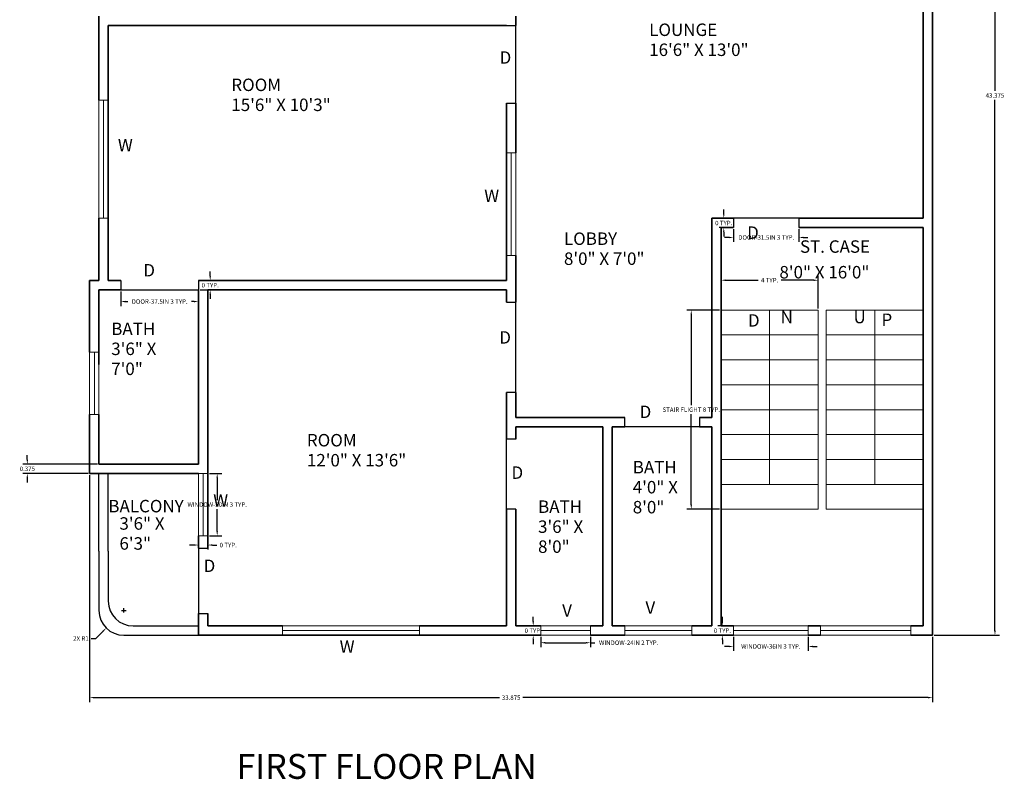
# Model space of a CAD drawing. Units: feet. Extents: x 60.2 to 151.6, y 170.7 to 222.6.
# Tile 2 of 3: x 112 to 151.6, y 170.7 to 201.2. Entities that reach past the tile are written whole.
import ezdxf

# ---------------------------------------------------------------- set-up
doc = ezdxf.new("R2010")
doc.units = ezdxf.units.FT
for name, color, linetype, lineweight in [('A-ANNO-DIMS', 7, 'Continuous', 13), ('A-ANNO-TEXT', 7, 'Continuous', 13), ('A-ANNO-TITL', 7, 'Continuous', 25), ('A-AREA-IDEN', 7, 'Continuous', 18), ('A-DOOR', 6, 'Continuous', 25), ('A-FLOR-BALC', 6, 'Continuous', 25), ('A-FLOR-STRS', 6, 'Continuous', 18), ('A-GLAZ', 240, 'Continuous', 18), ('A-WALL', 175, 'Continuous', 35)]:
    doc.layers.add(name, color=color, linetype=linetype, lineweight=lineweight)
doc.styles.get("Standard").update_dxf_attribs({"font": 'arial.ttf'})
doc.dimstyles.get("Standard").update_dxf_attribs({"dimtxt": 0.18, "dimasz": 0.18, "dimexe": 0.18, "dimexo": 0.0625, "dimgap": 0.09, "dimtad": 0, "dimtih": 1, "dimtoh": 1, "dimdec": 4, "dimzin": 0, "dimdsep": 46, "dimtxsty": 'Standard', "dimcen": 0.09, "dimadec": 0, "dimazin": 0, "dimtfac": 1, "dimtdec": 4, "dimtofl": 0, "dimtmove": 0, "dimatfit": 3, "dimfxl": 1, "dimtolj": 1, "dimtzin": 0, "dimarcsym": 0})

# ---------------------------------------------------------------- blocks, each defined once
blk = doc.blocks.new('DOOR-36IN')
for p, q in [((0, 0.375), (3, 0.375)), ((0, 0), (0, 0.375)), ((3, 0.375), (3, 0))]:
    blk.add_line(p, q)
blk = doc.blocks.new('DOOR-31_5IN')
for p, q in [((0, 2.625), (0, 0)), ((0, 2.625), (0.375, 2.625)), ((0, 0), (0.375, 0))]:
    blk.add_line(p, q)
blk = doc.blocks.new('DOOR-37_5IN')
for p, q in [((0, 0.375), (0, 0)), ((0, 0), (3.125, 0)), ((3.125, 0.375), (3.125, 0))]:
    blk.add_line(p, q)
blk = doc.blocks.new('WINDOW-24IN')
for p, q in [((0, 2), (0.375, 2)), ((0, 2), (0, 0)), ((0.188, 2), (0.188, 0)), ((0.375, 2), (0.375, 0)), ((0, 0), (0.375, 0))]:
    blk.add_line(p, q)
blk = doc.blocks.new('WINDOW-66IN')
for p, q in [((0.375, 5.5), (0, 5.5)), ((0, 0), (0, 5.5)), ((0.188, 5.5), (0.188, 0)), ((0.375, 0), (0.375, 5.5)), ((0.375, 0), (0, 0))]:
    blk.add_line(p, q)
blk = doc.blocks.new('WINDOW-30IN')
for p, q in [((0, 2.5), (0, 0)), ((0, 2.5), (0.375, 2.5)), ((0.188, 2.5), (0.188, 0)), ((0.375, 2.5), (0.375, 0)), ((0.375, 0.5), (0.375, 0)), ((0.375, 0), (0, 0))]:
    blk.add_line(p, q)
blk = doc.blocks.new('STAIR-FLIGHT-9-TREADS')
for p, q in [((0, 8), (3.9, 8)), ((1.95, 8), (1.95, 1)), ((3.9, 8), (3.9, 0)), ((0, 7), (3.9, 7)), ((0, 6), (3.9, 6)), ((0, 5), (3.9, 5)), ((0, 4), (3.9, 4)), ((0, 3), (3.9, 3)), ((0, 2), (3.9, 2)), ((0, 1), (3.9, 1)), ((0, 0), (3.9, 0))]:
    blk.add_line(p, q)
blk = doc.blocks.new('WINDOW-36IN')
for p, q in [((0, 0), (0, 3)), ((0, 3), (0.375, 3)), ((0.188, 3), (0.188, 0)), ((0.375, 3), (0.375, 0)), ((0.375, 0), (0, 0))]:
    blk.add_line(p, q)
blk = doc.blocks.new('*D20')
at = {"layer": 'A-ANNO-DIMS', "color": 0, "lineweight": -2, "transparency": 16777216}
for p, q in [((140.714, 192.831), (140.714, 192.319)), ((143.339, 192.831), (143.339, 192.319)), ((140.534, 192.499), (140.354, 192.499)), ((143.519, 192.499), (143.699, 192.499))]:
    blk.add_line(p, q, dxfattribs=at)
at = {"layer": 'A-ANNO-DIMS', "color": 0, "transparency": 16777216}
for points in [[(140.534, 192.529), (140.534, 192.469), (140.714, 192.499)], [(143.519, 192.529), (143.519, 192.469), (143.339, 192.499)]]:
    blk.add_solid(points, dxfattribs=at)
at = {"layer": 'Defpoints', "color": 0, "transparency": 16777216}
for p in [(140.714, 192.893), (143.339, 192.893), (143.339, 192.499)]:
    blk.add_point(p, dxfattribs=at)
at = {"layer": 'A-ANNO-DIMS', "color": 0, "transparency": 16777216, "insert": (142.027, 192.499), "char_height": 0.18, "attachment_point": 5}
blk.add_mtext('\\A1;DOOR-31.5IN 3 TYP.', dxfattribs=at)
blk = doc.blocks.new('*D21')
at = {"layer": 'A-ANNO-DIMS', "color": 0, "lineweight": -2, "transparency": 16777216}
for p, q in [((140.32, 193.448), (140.32, 193.628)), ((140.652, 193.268), (140.14, 193.268)), ((140.652, 192.893), (140.14, 192.893)), ((140.32, 192.713), (140.32, 192.533))]:
    blk.add_line(p, q, dxfattribs=at)
at = {"layer": 'A-ANNO-DIMS', "color": 0, "transparency": 16777216}
for points in [[(140.29, 193.448), (140.35, 193.448), (140.32, 193.268)], [(140.29, 192.713), (140.35, 192.713), (140.32, 192.893)]]:
    blk.add_solid(points, dxfattribs=at)
at = {"layer": 'Defpoints', "color": 0, "transparency": 16777216}
for p in [(140.714, 193.268), (140.32, 192.893), (140.714, 192.893)]:
    blk.add_point(p, dxfattribs=at)
at = {"layer": 'A-ANNO-DIMS', "color": 0, "transparency": 16777216, "insert": (140.32, 193.081), "char_height": 0.18, "attachment_point": 5}
blk.add_mtext('\\A1;0 TYP.', dxfattribs=at)
blk = doc.blocks.new('*D22')
at = {"layer": 'A-ANNO-DIMS', "color": 0, "lineweight": -2, "transparency": 16777216}
for p, q in [((116.089, 190.331), (116.089, 189.744)), ((119.214, 190.331), (119.214, 189.744)), ((116.269, 189.924), (116.374, 189.924)), ((119.034, 189.924), (118.93, 189.924))]:
    blk.add_line(p, q, dxfattribs=at)
at = {"layer": 'A-ANNO-DIMS', "color": 0, "transparency": 16777216}
for points in [[(116.269, 189.954), (116.269, 189.894), (116.089, 189.924)], [(119.034, 189.954), (119.034, 189.894), (119.214, 189.924)]]:
    blk.add_solid(points, dxfattribs=at)
at = {"layer": 'Defpoints', "color": 0, "transparency": 16777216}
for p in [(116.089, 190.393), (119.214, 190.393), (119.214, 189.924)]:
    blk.add_point(p, dxfattribs=at)
at = {"layer": 'A-ANNO-DIMS', "color": 0, "transparency": 16777216, "insert": (117.652, 189.924), "char_height": 0.18, "attachment_point": 5}
blk.add_mtext('\\A1;DOOR-37.5IN 3 TYP.', dxfattribs=at)
blk = doc.blocks.new('*D23')
at = {"layer": 'A-ANNO-DIMS', "color": 0, "lineweight": -2, "transparency": 16777216}
for p, q in [((119.683, 190.948), (119.683, 191.128)), ((119.277, 190.768), (119.863, 190.768)), ((119.277, 190.393), (119.863, 190.393)), ((119.683, 190.213), (119.683, 190.033))]:
    blk.add_line(p, q, dxfattribs=at)
at = {"layer": 'A-ANNO-DIMS', "color": 0, "transparency": 16777216}
for points in [[(119.653, 190.948), (119.713, 190.948), (119.683, 190.768)], [(119.653, 190.213), (119.713, 190.213), (119.683, 190.393)]]:
    blk.add_solid(points, dxfattribs=at)
at = {"layer": 'Defpoints', "color": 0, "transparency": 16777216}
for p in [(119.214, 190.768), (119.683, 190.768), (119.214, 190.393)]:
    blk.add_point(p, dxfattribs=at)
at = {"layer": 'A-ANNO-DIMS', "color": 0, "transparency": 16777216, "insert": (119.683, 190.581), "char_height": 0.18, "attachment_point": 5}
blk.add_mtext('\\A1;0 TYP.', dxfattribs=at)
blk = doc.blocks.new('*D24')
at = {"layer": 'A-ANNO-DIMS', "color": 0, "lineweight": -2, "transparency": 16777216}
for p, q in [((132.964, 176.456), (132.964, 176.038)), ((133.144, 176.218), (134.784, 176.218)), ((134.964, 176.456), (134.964, 176.038)), ((134.964, 176.218), (135.144, 176.218))]:
    blk.add_line(p, q, dxfattribs=at)
at = {"layer": 'A-ANNO-DIMS', "color": 0, "transparency": 16777216}
for points in [[(133.144, 176.248), (133.144, 176.188), (132.964, 176.218)], [(134.784, 176.248), (134.784, 176.188), (134.964, 176.218)]]:
    blk.add_solid(points, dxfattribs=at)
at = {"layer": 'Defpoints', "color": 0, "transparency": 16777216}
for p in [(132.964, 176.518), (134.964, 176.518), (134.964, 176.218)]:
    blk.add_point(p, dxfattribs=at)
at = {"layer": 'A-ANNO-DIMS', "color": 0, "transparency": 16777216, "insert": (136.5, 176.218), "char_height": 0.18, "attachment_point": 5}
blk.add_mtext('\\A1;WINDOW-24IN 2 TYP.', dxfattribs=at)
blk = doc.blocks.new('*D25')
at = {"layer": 'A-ANNO-DIMS', "color": 0, "lineweight": -2, "transparency": 16777216}
for p, q in [((132.902, 176.893), (132.484, 176.893)), ((132.664, 177.073), (132.664, 177.253)), ((132.902, 176.518), (132.484, 176.518)), ((132.664, 176.338), (132.664, 176.158))]:
    blk.add_line(p, q, dxfattribs=at)
at = {"layer": 'A-ANNO-DIMS', "color": 0, "transparency": 16777216}
for points in [[(132.634, 177.073), (132.694, 177.073), (132.664, 176.893)], [(132.634, 176.338), (132.694, 176.338), (132.664, 176.518)]]:
    blk.add_solid(points, dxfattribs=at)
at = {"layer": 'Defpoints', "color": 0, "transparency": 16777216}
for p in [(132.964, 176.893), (132.664, 176.518), (132.964, 176.518)]:
    blk.add_point(p, dxfattribs=at)
at = {"layer": 'A-ANNO-DIMS', "color": 0, "transparency": 16777216, "insert": (132.664, 176.706), "char_height": 0.18, "attachment_point": 5}
blk.add_mtext('\\A1;0 TYP.', dxfattribs=at)
blk = doc.blocks.new('*D26')
at = {"layer": 'A-ANNO-DIMS', "color": 0, "lineweight": -2, "transparency": 16777216}
for p, q in [((119.652, 183.018), (120.144, 183.018)), ((119.964, 182.838), (119.964, 181.951)), ((119.964, 180.698), (119.964, 181.585)), ((119.652, 180.518), (120.144, 180.518))]:
    blk.add_line(p, q, dxfattribs=at)
at = {"layer": 'A-ANNO-DIMS', "color": 0, "transparency": 16777216}
for points in [[(119.934, 182.838), (119.994, 182.838), (119.964, 183.018)], [(119.934, 180.698), (119.994, 180.698), (119.964, 180.518)]]:
    blk.add_solid(points, dxfattribs=at)
at = {"layer": 'Defpoints', "color": 0, "transparency": 16777216}
for p in [(119.589, 183.018), (119.964, 183.018), (119.589, 180.518)]:
    blk.add_point(p, dxfattribs=at)
at = {"layer": 'A-ANNO-DIMS', "color": 0, "transparency": 16777216, "insert": (119.964, 181.768), "char_height": 0.18, "attachment_point": 5}
blk.add_mtext('\\A1;WINDOW-30IN 3 TYP.', dxfattribs=at)
blk = doc.blocks.new('*D27')
at = {"layer": 'A-ANNO-DIMS', "color": 0, "lineweight": -2, "transparency": 16777216}
for p, q in [((119.214, 180.456), (119.214, 179.963)), ((119.589, 180.456), (119.589, 179.963)), ((119.034, 180.143), (118.854, 180.143)), ((119.769, 180.143), (119.949, 180.143))]:
    blk.add_line(p, q, dxfattribs=at)
at = {"layer": 'A-ANNO-DIMS', "color": 0, "transparency": 16777216}
for points in [[(119.034, 180.173), (119.034, 180.113), (119.214, 180.143)], [(119.769, 180.173), (119.769, 180.113), (119.589, 180.143)]]:
    blk.add_solid(points, dxfattribs=at)
at = {"layer": 'Defpoints', "color": 0, "transparency": 16777216}
for p in [(119.214, 180.518), (119.589, 180.518), (119.589, 180.143)]:
    blk.add_point(p, dxfattribs=at)
at = {"layer": 'A-ANNO-DIMS', "color": 0, "transparency": 16777216, "insert": (120.407, 180.143), "char_height": 0.18, "attachment_point": 5}
blk.add_mtext('\\A1;0 TYP.', dxfattribs=at)
blk = doc.blocks.new('*D28')
at = {"layer": 'A-ANNO-DIMS', "color": 0, "lineweight": -2, "transparency": 16777216}
for p, q in [((140.714, 176.456), (140.714, 175.888)), ((143.714, 176.456), (143.714, 175.888)), ((140.534, 176.068), (140.354, 176.068)), ((143.894, 176.068), (144.074, 176.068))]:
    blk.add_line(p, q, dxfattribs=at)
at = {"layer": 'A-ANNO-DIMS', "color": 0, "transparency": 16777216}
for points in [[(140.534, 176.098), (140.534, 176.038), (140.714, 176.068)], [(143.894, 176.098), (143.894, 176.038), (143.714, 176.068)]]:
    blk.add_solid(points, dxfattribs=at)
at = {"layer": 'Defpoints', "color": 0, "transparency": 16777216}
for p in [(140.714, 176.518), (143.714, 176.518), (143.714, 176.068)]:
    blk.add_point(p, dxfattribs=at)
at = {"layer": 'A-ANNO-DIMS', "color": 0, "transparency": 16777216, "insert": (142.214, 176.068), "char_height": 0.18, "attachment_point": 5}
blk.add_mtext('\\A1;WINDOW-36IN 3 TYP.', dxfattribs=at)
blk = doc.blocks.new('*D29')
at = {"layer": 'A-ANNO-DIMS', "color": 0, "lineweight": -2, "transparency": 16777216}
for p, q in [((140.652, 176.893), (140.084, 176.893)), ((140.264, 177.073), (140.264, 177.253)), ((140.652, 176.518), (140.084, 176.518)), ((140.264, 176.338), (140.264, 176.158))]:
    blk.add_line(p, q, dxfattribs=at)
at = {"layer": 'A-ANNO-DIMS', "color": 0, "transparency": 16777216}
for points in [[(140.234, 177.073), (140.294, 177.073), (140.264, 176.893)], [(140.234, 176.338), (140.294, 176.338), (140.264, 176.518)]]:
    blk.add_solid(points, dxfattribs=at)
at = {"layer": 'Defpoints', "color": 0, "transparency": 16777216}
for p in [(140.714, 176.893), (140.264, 176.518), (140.714, 176.518)]:
    blk.add_point(p, dxfattribs=at)
at = {"layer": 'A-ANNO-DIMS', "color": 0, "transparency": 16777216, "insert": (140.264, 176.706), "char_height": 0.18, "attachment_point": 5}
blk.add_mtext('\\A1;0 TYP.', dxfattribs=at)
blk = doc.blocks.new('*D36')
at = {"layer": 'A-ANNO-DIMS', "color": 0, "lineweight": -2, "transparency": 16777216}
for p, q in [((140.152, 189.581), (138.834, 189.581)), ((139.014, 189.401), (139.014, 185.764)), ((139.014, 181.761), (139.014, 185.398)), ((140.152, 181.581), (138.834, 181.581))]:
    blk.add_line(p, q, dxfattribs=at)
at = {"layer": 'A-ANNO-DIMS', "color": 0, "transparency": 16777216}
for points in [[(138.984, 189.401), (139.044, 189.401), (139.014, 189.581)], [(138.984, 181.761), (139.044, 181.761), (139.014, 181.581)]]:
    blk.add_solid(points, dxfattribs=at)
at = {"layer": 'Defpoints', "color": 0, "transparency": 16777216}
for p in [(139.014, 189.581), (140.214, 189.581), (140.214, 181.581)]:
    blk.add_point(p, dxfattribs=at)
at = {"layer": 'A-ANNO-DIMS', "color": 0, "transparency": 16777216, "insert": (139.014, 185.581), "char_height": 0.18, "attachment_point": 5}
blk.add_mtext('\\A1;STAIR FLIGHT 8 TYP.', dxfattribs=at)
blk = doc.blocks.new('*D37')
at = {"layer": 'A-ANNO-DIMS', "color": 0, "lineweight": -2, "transparency": 16777216}
for p, q in [((140.214, 189.643), (140.214, 190.961)), ((140.394, 190.781), (141.702, 190.781)), ((143.934, 190.781), (142.626, 190.781)), ((144.114, 189.643), (144.114, 190.961))]:
    blk.add_line(p, q, dxfattribs=at)
at = {"layer": 'A-ANNO-DIMS', "color": 0, "transparency": 16777216}
for points in [[(140.394, 190.811), (140.394, 190.751), (140.214, 190.781)], [(143.934, 190.811), (143.934, 190.751), (144.114, 190.781)]]:
    blk.add_solid(points, dxfattribs=at)
at = {"layer": 'Defpoints', "color": 0, "transparency": 16777216}
for p in [(144.114, 190.781), (140.214, 189.581), (144.114, 189.581)]:
    blk.add_point(p, dxfattribs=at)
at = {"layer": 'A-ANNO-DIMS', "color": 0, "transparency": 16777216, "insert": (142.164, 190.781), "char_height": 0.18, "attachment_point": 5}
blk.add_mtext('\\A1;4 TYP.', dxfattribs=at)
blk = doc.blocks.new('*D44')
at = {"layer": 'A-ANNO-DIMS', "color": 0, "lineweight": -2, "transparency": 16777216}
for p, q in [((114.839, 182.956), (114.839, 173.833)), ((148.714, 176.456), (148.714, 173.833)), ((115.019, 174.013), (131.312, 174.013)), ((148.534, 174.013), (132.241, 174.013))]:
    blk.add_line(p, q, dxfattribs=at)
at = {"layer": 'A-ANNO-DIMS', "color": 0, "transparency": 16777216}
for points in [[(115.019, 174.043), (115.019, 173.983), (114.839, 174.013)], [(148.534, 174.043), (148.534, 173.983), (148.714, 174.013)]]:
    blk.add_solid(points, dxfattribs=at)
at = {"layer": 'Defpoints', "color": 0, "transparency": 16777216}
for p in [(114.839, 183.018), (148.714, 176.518), (148.714, 174.013)]:
    blk.add_point(p, dxfattribs=at)
at = {"layer": 'A-ANNO-DIMS', "color": 0, "transparency": 16777216, "insert": (131.777, 174.013), "char_height": 0.18, "attachment_point": 5}
blk.add_mtext('\\A1;33.875', dxfattribs=at)
blk = doc.blocks.new('*D45')
at = {"layer": 'A-ANNO-DIMS', "color": 0, "lineweight": -2, "transparency": 16777216}
for p, q in [((148.777, 219.893), (151.399, 219.893)), ((151.219, 219.713), (151.219, 198.388)), ((151.219, 176.698), (151.219, 198.024)), ((148.777, 176.518), (151.399, 176.518))]:
    blk.add_line(p, q, dxfattribs=at)
at = {"layer": 'A-ANNO-DIMS', "color": 0, "transparency": 16777216}
for points in [[(151.189, 219.713), (151.249, 219.713), (151.219, 219.893)], [(151.189, 176.698), (151.249, 176.698), (151.219, 176.518)]]:
    blk.add_solid(points, dxfattribs=at)
at = {"layer": 'Defpoints', "color": 0, "transparency": 16777216}
for p in [(148.714, 219.893), (151.219, 219.893), (148.714, 176.518)]:
    blk.add_point(p, dxfattribs=at)
at = {"layer": 'A-ANNO-DIMS', "color": 0, "transparency": 16777216, "insert": (151.219, 198.206), "char_height": 0.18, "attachment_point": 5}
blk.add_mtext('\\A1;43.375', dxfattribs=at)
blk = doc.blocks.new('*D49')
at = {"layer": 'A-ANNO-DIMS', "color": 0, "lineweight": -2, "transparency": 16777216}
for p, q in [((112.334154, 183.5732), (112.334154, 183.7532)), ((115.151654, 183.3932), (112.154154, 183.3932)), ((114.776654, 183.0182), (112.154154, 183.0182)), ((112.334154, 182.8382), (112.334154, 182.6582))]:
    blk.add_line(p, q, dxfattribs=at)
at = {"layer": 'A-ANNO-DIMS', "color": 0, "transparency": 16777216}
for points in [[(112.304154, 183.5732), (112.364154, 183.5732), (112.334154, 183.3932)], [(112.304154, 182.8382), (112.364154, 182.8382), (112.334154, 183.0182)]]:
    blk.add_solid(points, dxfattribs=at)
at = {"layer": 'Defpoints', "color": 0, "transparency": 16777216}
for p in [(112.334154, 183.3932), (115.214154, 183.3932), (114.839154, 183.0182)]:
    blk.add_point(p, dxfattribs=at)
at = {"layer": 'A-ANNO-DIMS', "color": 0, "transparency": 16777216, "insert": (112.334154, 183.2057), "char_height": 0.18, "attachment_point": 5}
blk.add_mtext('\\A1;0.375', dxfattribs=at)
blk = doc.blocks.new('*D50')
at = {"layer": 'A-ANNO-DIMS', "color": 0, "lineweight": -2, "transparency": 16777216}
for p, q in [((116.124, 177.518), (116.304, 177.518)), ((116.214, 177.428), (116.214, 177.608)), ((115.083, 176.387), (115.38, 176.684)), ((114.903, 176.387), (115.083, 176.387))]:
    blk.add_line(p, q, dxfattribs=at)
at = {"layer": 'A-ANNO-DIMS', "color": 0, "transparency": 16777216}
blk.add_solid([(115.359, 176.705), (115.401, 176.663), (115.507, 176.811)], dxfattribs=at)
at = {"layer": 'Defpoints', "color": 0, "transparency": 16777216}
for p in [(116.214, 177.518), (115.507, 176.811)]:
    blk.add_point(p, dxfattribs=at)
at = {"layer": 'A-ANNO-DIMS', "color": 0, "transparency": 16777216, "insert": (114.49, 176.387), "char_height": 0.18, "attachment_point": 5}
blk.add_mtext('\\A1;2X R1', dxfattribs=at)

msp = doc.modelspace()

# ---------------------------------------------------------------- linework, layer by layer
at = {"layer": 'A-DOOR'}
for p, q in [((131.5892, 189.8932), (131.9642, 189.8932)), ((131.9642, 186.2682), (131.9642, 189.8932)), ((131.9642, 186.2682), (131.5892, 186.2682)), ((131.9642, 184.3932), (131.5892, 184.3932)), ((131.5892, 181.5807), (131.5892, 184.3932)), ((131.9642, 181.5807), (131.5892, 181.5807))]:
    msp.add_line(p, q, dxfattribs=at)
at = {"layer": 'A-FLOR-BALC'}
for p, q in [((115.2142, 179.8932), (115.2142, 183.0182)), ((115.5892, 179.8932), (115.5892, 183.0182)), ((115.2142, 179.8932), (115.2142, 177.5182)), ((115.5892, 179.8932), (115.5892, 177.8932)), ((116.5892, 176.8932), (119.2142, 176.8932)), ((116.2142, 176.5182), (119.2142, 176.5182))]:
    msp.add_line(p, q, dxfattribs=at)
for centre in [(116.5892, 177.8932), (116.2142, 177.5182)]:
    msp.add_arc(centre, 1, 180, 270, dxfattribs=at)
at = {"layer": 'A-FLOR-STRS'}
msp.add_line((148.3392, 187.5807), (144.4392, 187.5807), dxfattribs=at)
at = {"layer": 'A-GLAZ'}
for p, q in [((115.5892, 198.0182), (115.2142, 198.0182)), ((115.2142, 193.2682), (115.2142, 198.0182)), ((115.4017, 198.0182), (115.4017, 193.2682)), ((115.5892, 198.0182), (115.5892, 193.2682)), ((131.5892, 191.7682), (131.5892, 195.8932)), ((131.5892, 195.8932), (131.9642, 195.8932)), ((131.7767, 195.8932), (131.7767, 191.7682)), ((131.9642, 191.7682), (131.9642, 195.8932)), ((115.2142, 193.2682), (115.5892, 193.2682)), ((131.5892, 191.7682), (131.9642, 191.7682)), ((136.3392, 176.8932), (136.3392, 176.5182)), ((136.3392, 176.8932), (139.0392, 176.8932)), ((139.0392, 176.8932), (139.0392, 176.5182)), ((140.7142, 176.8932), (143.2142, 176.8932)), ((144.2142, 176.8932), (144.2142, 176.5182)), ((144.2142, 176.8932), (147.8392, 176.8932)), ((147.8392, 176.8932), (147.8392, 176.5182)), ((136.3392, 176.7057), (139.0392, 176.7057)), ((136.3392, 176.5182), (139.0392, 176.5182)), ((143.2142, 176.5182), (143.7142, 176.5182)), ((144.2142, 176.7057), (147.8392, 176.7057)), ((144.2142, 176.5182), (147.8392, 176.5182))]:
    msp.add_line(p, q, dxfattribs=at)
at = {"layer": 'A-WALL'}
for p, q in [((148.7142, 216.0182), (148.7142, 179.8932)), ((148.3392, 205.6432), (148.3392, 193.2682)), ((115.2142, 198.0182), (115.2142, 201.3932)), ((131.5892, 201.0182), (115.5892, 201.0182)), ((115.5892, 201.0182), (115.5892, 198.0182)), ((115.5892, 190.7682), (115.5892, 201.0182)), ((115.5892, 201.0182), (115.5892, 199.0182)), ((119.7142, 201.0182), (127.2142, 201.0182)), ((127.5892, 201.0182), (131.5892, 201.0182)), ((131.9642, 201.3932), (131.9642, 201.0182)), ((115.5892, 199.0182), (115.5892, 198.0182)), ((131.5892, 190.7682), (131.5892, 197.8932)), ((131.9642, 197.3932), (131.9642, 197.8932)), ((131.9642, 195.8932), (131.9642, 197.8932)), ((131.9642, 195.8932), (131.9642, 197.3932)), ((115.2142, 190.7682), (115.2142, 193.2682)), ((115.2142, 192.7682), (115.2142, 193.2682)), ((115.5892, 193.2682), (115.5892, 190.7682)), ((140.2142, 193.2682), (139.8392, 193.2682)), ((139.8392, 193.2682), (139.8392, 192.8932)), ((140.2142, 193.2682), (140.7142, 193.2682)), ((148.3392, 193.2682), (143.3392, 193.2682)), ((143.3392, 193.2682), (148.2142, 193.2682)), ((148.2142, 193.2682), (148.3142, 193.2682)), ((148.3142, 193.2682), (148.3392, 193.2682)), ((115.2142, 190.7682), (115.2142, 192.7682)), ((139.8392, 185.2682), (139.8392, 192.8932)), ((140.2142, 176.8932), (140.2142, 192.8932)), ((140.2142, 192.8932), (140.7142, 192.8932)), ((140.2142, 192.8932), (140.7142, 192.8932)), ((143.3392, 192.8932), (148.2142, 192.8932)), ((148.2142, 192.8932), (148.3392, 192.8932)), ((148.3392, 192.8932), (148.3392, 180.2682)), ((131.5892, 190.7682), (131.5892, 191.7682)), ((131.9642, 190.7682), (131.9642, 191.7682)), ((114.8392, 190.3932), (114.8392, 190.7682)), ((114.8392, 190.7682), (115.2142, 190.7682)), ((115.5892, 190.7682), (116.0892, 190.7682)), ((115.5892, 190.7682), (116.0892, 190.7682)), ((119.2142, 190.7682), (131.5892, 190.7682)), ((131.9642, 189.8932), (131.9642, 190.7682)), ((114.8392, 190.3932), (114.8392, 187.8932)), ((115.2142, 190.3932), (115.2142, 187.8932)), ((115.2142, 190.3932), (115.5892, 190.3932)), ((115.2142, 190.3932), (115.2142, 188.3932)), ((115.5892, 190.3932), (116.0892, 190.3932)), ((119.2142, 190.3932), (119.2142, 183.3932)), ((131.5892, 190.3932), (119.5892, 190.3932)), ((119.5892, 190.3932), (119.5892, 180.0182)), ((119.5892, 190.3932), (131.5892, 190.3932)), ((131.5892, 190.3932), (131.5892, 189.8932)), ((131.5892, 189.8932), (131.5892, 190.3932)), ((131.9642, 189.8932), (131.9642, 190.3932)), ((115.2142, 188.3932), (115.2142, 187.3932)), ((131.5892, 184.3932), (131.5892, 186.2682)), ((131.9642, 185.2682), (131.9642, 186.2682)), ((131.9642, 185.2682), (131.9642, 186.2682)), ((114.8392, 185.3932), (114.8392, 183.3932)), ((115.2142, 183.3932), (115.2142, 185.3932)), ((115.2142, 185.3932), (115.2142, 183.3932)), ((131.9642, 185.2682), (135.4642, 185.2682)), ((135.4642, 185.2682), (135.8392, 185.2682)), ((135.8392, 185.2682), (136.3392, 185.2682)), ((135.8392, 185.2682), (136.3392, 185.2682)), ((139.8392, 185.2682), (139.3392, 185.2682)), ((139.3392, 185.2682), (139.8392, 185.2682)), ((131.9642, 184.8932), (135.4642, 184.8932)), ((131.9642, 184.8932), (131.9642, 184.3932)), ((131.9642, 184.3932), (131.9642, 184.8932)), ((131.9642, 184.3932), (131.9642, 184.8932)), ((135.4642, 184.8932), (135.4642, 176.8932)), ((135.8392, 184.8932), (135.8392, 176.8932)), ((135.8392, 176.8932), (135.8392, 184.8932)), ((135.8392, 184.8932), (136.3392, 184.8932)), ((139.3392, 184.8932), (139.8392, 184.8932)), ((139.8392, 184.8932), (139.8392, 176.8932)), ((139.8392, 176.8932), (139.8392, 184.8932)), ((140.2142, 184.8932), (140.2142, 176.8932)), ((114.8392, 183.3932), (114.8392, 183.0182)), ((115.2142, 183.3932), (119.2142, 183.3932)), ((114.8392, 183.0182), (115.5892, 183.0182)), ((115.5892, 183.0182), (119.2142, 183.0182)), ((131.5892, 176.8932), (131.5892, 181.5807)), ((131.9642, 176.8932), (131.9642, 181.5807)), ((131.9642, 176.8932), (131.9642, 181.5807)), ((119.5892, 180.0182), (119.5892, 181.0182)), ((119.2142, 180.5182), (119.2142, 180.0182)), ((119.2142, 180.5182), (119.2142, 180.0182)), ((119.5892, 180.0182), (119.5892, 180.5182)), ((119.5892, 180.5182), (119.5892, 180.0182)), ((148.3392, 176.8932), (148.3392, 180.2682)), ((148.7142, 176.5182), (148.7142, 179.8932)), ((119.2142, 176.8932), (119.2142, 177.3932)), ((119.2142, 177.3932), (119.2142, 176.8932)), ((119.5892, 177.3932), (119.5892, 176.8932)), ((119.2142, 176.8932), (119.2142, 176.5182)), ((119.5892, 176.8932), (122.5892, 176.8932)), ((119.5892, 176.8932), (122.5892, 176.8932)), ((128.5892, 176.8932), (128.0892, 176.8932)), ((128.0892, 176.8932), (131.5892, 176.8932)), ((131.5892, 176.8932), (128.5892, 176.8932)), ((131.9642, 176.8932), (132.9642, 176.8932)), ((131.9642, 176.8932), (132.9642, 176.8932)), ((135.4642, 176.8932), (134.9642, 176.8932)), ((134.9642, 176.8932), (135.4642, 176.8932)), ((135.8392, 176.8932), (136.3392, 176.8932)), ((135.8392, 176.8932), (136.3392, 176.8932)), ((139.8392, 176.8932), (139.0392, 176.8932)), ((139.0392, 176.8932), (139.8392, 176.8932)), ((140.2142, 176.8932), (140.7142, 176.8932)), ((140.2142, 176.8932), (140.7142, 176.8932)), ((143.7142, 176.8932), (144.2142, 176.8932)), ((143.7142, 176.8932), (144.2142, 176.8932)), ((148.3392, 176.8932), (147.8392, 176.8932)), ((147.8392, 176.8932), (148.3392, 176.8932)), ((119.2142, 176.5182), (119.5892, 176.5182)), ((119.5892, 176.5182), (131.5892, 176.5182)), ((119.5892, 176.5182), (122.5892, 176.5182)), ((128.0892, 176.5182), (132.9642, 176.5182)), ((134.9642, 176.5182), (136.3392, 176.5182)), ((139.0392, 176.5182), (140.7142, 176.5182)), ((143.7142, 176.5182), (144.2142, 176.5182)), ((147.8392, 176.5182), (148.7142, 176.5182))]:
    msp.add_line(p, q, dxfattribs=at)

# ---------------------------------------------------------------- block references
at = {"layer": 'A-DOOR'}
for name, p, rotation in [('DOOR-37_5IN', (131.9644, 197.893), 90.00000000000003), ('DOOR-31_5IN', (140.714, 193.2684), 270), ('DOOR-36IN', (139.3394, 185.2684), 180)]:
    msp.add_blockref(name, p, dxfattribs=dict(at, rotation=rotation))
for name, p in [('DOOR-37_5IN', (116.089, 190.393)), ('DOOR-31_5IN', (119.214, 177.393))]:
    msp.add_blockref(name, p, dxfattribs=at)
at = {"layer": 'A-FLOR-STRS'}
msp.add_blockref('STAIR-FLIGHT-9-TREADS', (140.214, 181.581), dxfattribs=at)
at = {"layer": 'A-FLOR-STRS', "extrusion": (0, 0, -1), "zscale": -1}
msp.add_blockref('STAIR-FLIGHT-9-TREADS', (-148.3393, 181.581), dxfattribs=at)
at = {"layer": 'A-GLAZ', "extrusion": (0, 0, -1), "zscale": -1, "rotation": 180}
msp.add_blockref('WINDOW-30IN', (-114.839, 187.8934), dxfattribs=at)
at = {"layer": 'A-GLAZ'}
msp.add_blockref('WINDOW-30IN', (119.214, 180.518), dxfattribs=at)
for name, p, rotation in [('WINDOW-66IN', (122.589, 176.8934), 270.0000000000014), ('WINDOW-24IN', (132.964, 176.8935), 270.0000000000025), ('WINDOW-36IN', (140.714, 176.8934), 269.9999999999992)]:
    msp.add_blockref(name, p, dxfattribs=dict(at, rotation=rotation))

# ---------------------------------------------------------------- texts
at = {"layer": 'A-ANNO-DIMS'}
for s, p in [('16\'6" X 13\'0"', (137.3238, 199.7898)), ('15\'6" X 10\'3"', (120.5319, 197.5775)), ('8\'0" X 7\'0"', (133.8987, 191.3966)), ('8\'0" X 16\'0"', (142.5571, 190.8527)), ('3\'6" X ', (115.7058, 187.7748)), ('7\'0"', (115.7058, 186.9716)), ('12\'0" X 13\'6"', (123.5684, 183.3005)), ('4\'0" X ', (136.6636, 182.2174)), ('8\'0"', (136.6636, 181.4142)), ('3\'6" X', (116.0357, 180.7587)), ('3\'6" X', (132.8582, 180.6309)), ('6\'3"', (116.0357, 179.9555)), ('8\'0"', (132.8582, 179.8276))]:
    msp.add_text(s, height=0.5, dxfattribs=at).set_placement(p)
at = {"layer": 'A-ANNO-TEXT'}
for s, p in [('D', (131.3121, 199.4787)), ('W', (115.973, 195.9612)), ('W', (130.6954, 193.9254)), ('D', (141.2596, 192.4438)), ('D', (116.995, 190.9321)), ('N', (142.6059, 189.0522)), ('U', (145.5353, 189.0522)), ('D', (141.2918, 188.9154)), ('P', (146.6578, 188.9428)), ('D', (131.3001, 188.2329)), ('D', (136.9383, 185.2447)), ('D', (131.7905, 182.8018)), ('W', (119.8036, 181.6853)), ('D', (119.4177, 179.0581)), ('V', (133.8272, 177.2615)), ('V', (137.1732, 177.3822)), ('W', (124.8849, 175.8125))]:
    msp.add_text(s, height=0.5, dxfattribs=at).set_placement(p)
at = {"layer": 'A-ANNO-TITL'}
msp.add_text('FIRST FLOOR PLAN', height=1, dxfattribs=at).set_placement((120.7404, 170.7492))
at = {"layer": 'A-AREA-IDEN'}
for s, p in [('LOUNGE', (137.3238, 200.593)), ('ROOM', (120.5319, 198.3808)), ('LOBBY', (133.8987, 192.1998)), ('ST. CASE', (143.3828, 191.8839)), ('BATH', (115.7058, 188.578)), ('ROOM', (123.5684, 184.1037)), ('BATH', (136.6636, 183.0206)), ('BALCONY', (115.5892, 181.4557)), ('BATH', (132.8582, 181.4341))]:
    msp.add_text(s, height=0.5, dxfattribs=at).set_placement(p)

# ---------------------------------------------------------------- dimensions: what is measured, and where the dimension line sits
at = {"layer": 'A-ANNO-DIMS'}
for base, p1, p2, picture, middle in [((151.2192, 219.8932), (148.7142, 176.5182), (148.7142, 219.8932), '*D45', (151.2192, 198.2057)), ((112.3342, 183.3932), (114.8392, 183.0182), (115.2142, 183.3932), '*D49', (112.3342, 183.2057))]:
    dim = msp.add_linear_dim(base=base, p1=p1, p2=p2, angle=90, dimstyle='Standard', override={"dimdec": 3, "dimlfac": 1, "dimrnd": 0, "dimzin": 0, "dimdsep": 46, "dimlunit": 2}, dxfattribs=at)
    dim.commit()
    dim.dimension.update_dxf_attribs({"geometry": picture, "text_midpoint": middle})
for base, p1, p2, angle, text, picture, middle in [((140.3204, 192.8932), (140.7142, 193.2682), (140.7142, 192.8932), 270, '<> TYP.', '*D21', (140.3204, 193.0807)), ((119.6829, 190.7682), (119.2142, 190.3932), (119.2142, 190.7682), 90, '<> TYP.', '*D23', (119.6829, 190.5807)), ((139.0142, 189.5807), (140.2142, 181.5807), (140.2142, 189.5807), 90, 'STAIR FLIGHT <> TYP.', '*D36', (139.0142, 185.5807)), ((119.9641535563, 183.0182003807), (119.5891535563, 180.5182003807), (119.5891535563, 183.0182003807), 90, 'WINDOW-30IN <> TYP.', '*D26', (119.9641535563, 181.7682003807)), ((132.6642, 176.5182), (132.9642, 176.8932), (132.9642, 176.5182), 270, '<> TYP.', '*D25', (132.6642, 176.7057)), ((140.2642, 176.5182), (140.7142, 176.8932), (140.7142, 176.5182), 270, '<> TYP.', '*D29', (140.2642, 176.7057)), ((134.9642, 176.2182), (132.9642, 176.5182), (134.9642, 176.5182), 0, 'WINDOW-24IN <> TYP.', '*D24', (136.5, 176.2182))]:
    dim = msp.add_linear_dim(base=base, p1=p1, p2=p2, angle=angle, text=text, dimstyle='Standard', override={"dimdec": 0, "dimlfac": 1, "dimrnd": 0, "dimzin": 0, "dimdsep": 46, "dimlunit": 2}, dxfattribs=at)
    dim.commit()
    dim.dimension.update_dxf_attribs({"geometry": picture, "text_midpoint": middle})
for base, p1, p2, text, picture, middle in [((143.3392, 192.4995), (140.7142, 192.8932), (143.3392, 192.8932), 'DOOR-31.5IN <> TYP.', '*D20', (142.0267, 192.4995)), ((144.1142, 190.7807), (140.2142, 189.5807), (144.1142, 189.5807), '<> TYP.', '*D37', (142.1642, 190.7807)), ((119.2142, 189.9245), (116.0892, 190.3932), (119.2142, 190.3932), 'DOOR-37.5IN <> TYP.', '*D22', (117.6517, 189.9245)), ((119.5892, 180.1432), (119.2142, 180.5182), (119.5892, 180.5182), '<> TYP.', '*D27', (120.4073, 180.1432)), ((143.7142, 176.0682), (140.7142, 176.5182), (143.7142, 176.5182), 'WINDOW-36IN <> TYP.', '*D28', (142.2142, 176.0682))]:
    dim = msp.add_linear_dim(base=base, p1=p1, p2=p2, text=text, dimstyle='Standard', override={"dimdec": 0, "dimlfac": 1, "dimrnd": 0, "dimzin": 0, "dimdsep": 46, "dimlunit": 2}, dxfattribs=at)
    dim.commit()
    dim.dimension.update_dxf_attribs({"geometry": picture, "text_midpoint": middle})
dim = msp.add_linear_dim(base=(148.7142, 174.0132), p1=(114.8392, 183.0182), p2=(148.7142, 176.5182), dimstyle='Standard', override={"dimdec": 3, "dimlfac": 1, "dimrnd": 0, "dimzin": 0, "dimdsep": 46, "dimlunit": 2}, dxfattribs=at)
dim.commit()
dim.dimension.update_dxf_attribs({"geometry": '*D44', "text_midpoint": (131.7767, 174.0132)})
dim = msp.add_radius_dim(center=(116.2142, 177.5182), mpoint=(115.5071, 176.8111), text='2X <>', dimstyle='Standard', override={"dimdec": 0, "dimlfac": 1, "dimrnd": 0, "dimzin": 0, "dimdsep": 46, "dimlunit": 2}, dxfattribs=at)
dim.commit()
dim.dimension.update_dxf_attribs({"geometry": '*D50', "text_midpoint": (114.4901, 176.3868), "dimtype": 164})

doc.saveas('drawing.dxf')
